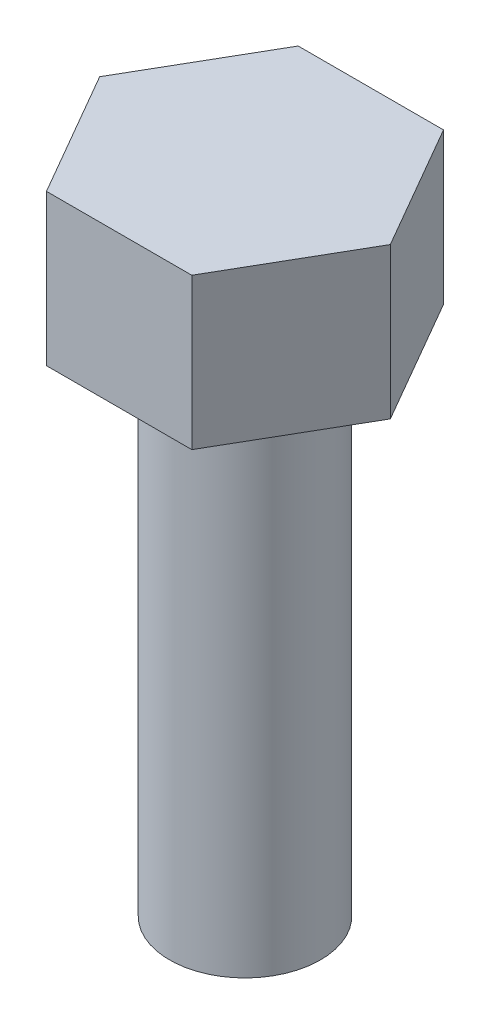
ISO-10303-21;
HEADER;
FILE_DESCRIPTION(('STEP AP214'),'2;1');
FILE_NAME('part.step','',(''),(''),'','','');
FILE_SCHEMA(('AUTOMOTIVE_DESIGN { 1 0 10303 214 1 1 1 1 }'));
ENDSEC;
DATA;
#1=APPLICATION_CONTEXT('core data for automotive mechanical design processes');
#2=APPLICATION_PROTOCOL_DEFINITION('international standard','automotive_design',2000,#1);
#3=PRODUCT_CONTEXT('',#1,'mechanical');
#4=PRODUCT('Part','Part','',(#3));
#5=PRODUCT_RELATED_PRODUCT_CATEGORY('part','',(#4));
#6=PRODUCT_DEFINITION_FORMATION('','',#4);
#7=PRODUCT_DEFINITION_CONTEXT('part definition',#1,'design');
#8=PRODUCT_DEFINITION('design','',#6,#7);
#9=PRODUCT_DEFINITION_SHAPE('','',#8);
#10=(LENGTH_UNIT() NAMED_UNIT(*) SI_UNIT(.MILLI.,.METRE.));
#11=(NAMED_UNIT(*) PLANE_ANGLE_UNIT() SI_UNIT($,.RADIAN.));
#12=(NAMED_UNIT(*) SI_UNIT($,.STERADIAN.) SOLID_ANGLE_UNIT());
#13=UNCERTAINTY_MEASURE_WITH_UNIT(LENGTH_MEASURE(1.E-05),#10,'distance_accuracy_value','');
#14=(GEOMETRIC_REPRESENTATION_CONTEXT(3) GLOBAL_UNCERTAINTY_ASSIGNED_CONTEXT((#13)) GLOBAL_UNIT_ASSIGNED_CONTEXT((#10,
#11,#12)) REPRESENTATION_CONTEXT('',''));
#15=CARTESIAN_POINT('',(0.,0.,0.));
#16=DIRECTION('',(0.,0.,1.));
#17=DIRECTION('',(1.,0.,0.));
#18=AXIS2_PLACEMENT_3D('',#15,#16,#17);
#19=CARTESIAN_POINT('',(1.44337567297406,3.,2.50000000000001));
#20=DIRECTION('',(-0.866025403784439,0.,-0.5));
#21=DIRECTION('',(-0.5,0.,0.866025403784439));
#22=AXIS2_PLACEMENT_3D('',#19,#20,#21);
#23=PLANE('',#22);
#24=DIRECTION('',(0.499999999999999,0.,-0.866025403784439));
#25=VECTOR('',#24,1.);
#26=CARTESIAN_POINT('',(1.44337567297406,0.,2.50000000000001));
#27=LINE('',#26,#25);
#28=CARTESIAN_POINT('',(1.44337567297406,0.,2.50000000000001));
#29=VERTEX_POINT('',#28);
#30=CARTESIAN_POINT('',(2.88675134594813,0.,0.));
#31=VERTEX_POINT('',#30);
#32=EDGE_CURVE('E124',#29,#31,#27,.T.);
#33=ORIENTED_EDGE('',*,*,#32,.T.);
#34=DIRECTION('',(0.,-1.,0.));
#35=VECTOR('',#34,1.);
#36=CARTESIAN_POINT('',(2.88675134594813,3.,0.));
#37=LINE('',#36,#35);
#38=CARTESIAN_POINT('',(2.88675134594813,3.,0.));
#39=VERTEX_POINT('',#38);
#40=EDGE_CURVE('E45',#39,#31,#37,.T.);
#41=ORIENTED_EDGE('',*,*,#40,.F.);
#42=DIRECTION('',(0.499999999999999,0.,-0.866025403784439));
#43=VECTOR('',#42,1.);
#44=CARTESIAN_POINT('',(1.44337567297406,3.,2.50000000000001));
#45=LINE('',#44,#43);
#46=CARTESIAN_POINT('',(1.44337567297406,3.,2.50000000000001));
#47=VERTEX_POINT('',#46);
#48=EDGE_CURVE('E138',#47,#39,#45,.T.);
#49=ORIENTED_EDGE('',*,*,#48,.F.);
#50=DIRECTION('',(0.,-1.,0.));
#51=VECTOR('',#50,1.);
#52=CARTESIAN_POINT('',(1.44337567297406,3.,2.50000000000001));
#53=LINE('',#52,#51);
#54=EDGE_CURVE('E123',#47,#29,#53,.T.);
#55=ORIENTED_EDGE('',*,*,#54,.T.);
#56=EDGE_LOOP('',(#33,#41,#49,#55));
#57=FACE_BOUND('',#56,.T.);
#58=ADVANCED_FACE('F39',(#57),#23,.F.);
#59=CARTESIAN_POINT('',(2.88675134594813,3.,0.));
#60=DIRECTION('',(-0.866025403784439,0.,0.5));
#61=DIRECTION('',(0.5,0.,0.866025403784439));
#62=AXIS2_PLACEMENT_3D('',#59,#60,#61);
#63=PLANE('',#62);
#64=DIRECTION('',(-0.5,0.,-0.866025403784438));
#65=VECTOR('',#64,1.);
#66=CARTESIAN_POINT('',(2.88675134594813,0.,0.));
#67=LINE('',#66,#65);
#68=CARTESIAN_POINT('',(1.44337567297406,0.,-2.50000000000001));
#69=VERTEX_POINT('',#68);
#70=EDGE_CURVE('E126',#31,#69,#67,.T.);
#71=ORIENTED_EDGE('',*,*,#70,.T.);
#72=DIRECTION('',(0.,-1.,0.));
#73=VECTOR('',#72,1.);
#74=CARTESIAN_POINT('',(1.44337567297406,3.,-2.50000000000001));
#75=LINE('',#74,#73);
#76=CARTESIAN_POINT('',(1.44337567297406,3.,-2.50000000000001));
#77=VERTEX_POINT('',#76);
#78=EDGE_CURVE('E137',#77,#69,#75,.T.);
#79=ORIENTED_EDGE('',*,*,#78,.F.);
#80=DIRECTION('',(-0.5,0.,-0.866025403784438));
#81=VECTOR('',#80,1.);
#82=CARTESIAN_POINT('',(2.88675134594813,3.,0.));
#83=LINE('',#82,#81);
#84=EDGE_CURVE('E94',#39,#77,#83,.T.);
#85=ORIENTED_EDGE('',*,*,#84,.F.);
#86=ORIENTED_EDGE('',*,*,#40,.T.);
#87=EDGE_LOOP('',(#71,#79,#85,#86));
#88=FACE_BOUND('',#87,.T.);
#89=ADVANCED_FACE('F145',(#88),#63,.F.);
#90=CARTESIAN_POINT('',(1.44337567297406,3.,-2.50000000000001));
#91=DIRECTION('',(0.,0.,1.));
#92=DIRECTION('',(1.,0.,0.));
#93=AXIS2_PLACEMENT_3D('',#90,#91,#92);
#94=PLANE('',#93);
#95=DIRECTION('',(-1.,0.,0.));
#96=VECTOR('',#95,1.);
#97=CARTESIAN_POINT('',(1.44337567297406,0.,-2.50000000000001));
#98=LINE('',#97,#96);
#99=CARTESIAN_POINT('',(-1.44337567297407,0.,-2.50000000000001));
#100=VERTEX_POINT('',#99);
#101=EDGE_CURVE('E131',#69,#100,#98,.T.);
#102=ORIENTED_EDGE('',*,*,#101,.T.);
#103=DIRECTION('',(0.,-1.,0.));
#104=VECTOR('',#103,1.);
#105=CARTESIAN_POINT('',(-1.44337567297407,3.,-2.50000000000001));
#106=LINE('',#105,#104);
#107=CARTESIAN_POINT('',(-1.44337567297407,3.,-2.50000000000001));
#108=VERTEX_POINT('',#107);
#109=EDGE_CURVE('E116',#108,#100,#106,.T.);
#110=ORIENTED_EDGE('',*,*,#109,.F.);
#111=DIRECTION('',(-1.,0.,0.));
#112=VECTOR('',#111,1.);
#113=CARTESIAN_POINT('',(1.44337567297406,3.,-2.50000000000001));
#114=LINE('',#113,#112);
#115=EDGE_CURVE('E110',#77,#108,#114,.T.);
#116=ORIENTED_EDGE('',*,*,#115,.F.);
#117=ORIENTED_EDGE('',*,*,#78,.T.);
#118=EDGE_LOOP('',(#102,#110,#116,#117));
#119=FACE_BOUND('',#118,.T.);
#120=ADVANCED_FACE('F147',(#119),#94,.F.);
#121=CARTESIAN_POINT('',(-1.44337567297407,3.,-2.50000000000001));
#122=DIRECTION('',(0.866025403784439,0.,0.5));
#123=DIRECTION('',(0.5,0.,-0.866025403784439));
#124=AXIS2_PLACEMENT_3D('',#121,#122,#123);
#125=PLANE('',#124);
#126=DIRECTION('',(-0.5,0.,0.866025403784439));
#127=VECTOR('',#126,1.);
#128=CARTESIAN_POINT('',(-1.44337567297407,0.,-2.50000000000001));
#129=LINE('',#128,#127);
#130=CARTESIAN_POINT('',(-2.88675134594813,0.,0.));
#131=VERTEX_POINT('',#130);
#132=EDGE_CURVE('E113',#100,#131,#129,.T.);
#133=ORIENTED_EDGE('',*,*,#132,.T.);
#134=DIRECTION('',(0.,-1.,0.));
#135=VECTOR('',#134,1.);
#136=CARTESIAN_POINT('',(-2.88675134594813,3.,0.));
#137=LINE('',#136,#135);
#138=CARTESIAN_POINT('',(-2.88675134594813,3.,0.));
#139=VERTEX_POINT('',#138);
#140=EDGE_CURVE('E115',#139,#131,#137,.T.);
#141=ORIENTED_EDGE('',*,*,#140,.F.);
#142=DIRECTION('',(-0.5,0.,0.866025403784439));
#143=VECTOR('',#142,1.);
#144=CARTESIAN_POINT('',(-1.44337567297407,3.,-2.50000000000001));
#145=LINE('',#144,#143);
#146=EDGE_CURVE('E101',#108,#139,#145,.T.);
#147=ORIENTED_EDGE('',*,*,#146,.F.);
#148=ORIENTED_EDGE('',*,*,#109,.T.);
#149=EDGE_LOOP('',(#133,#141,#147,#148));
#150=FACE_BOUND('',#149,.T.);
#151=ADVANCED_FACE('F114',(#150),#125,.F.);
#152=CARTESIAN_POINT('',(-2.88675134594813,3.,0.));
#153=DIRECTION('',(0.866025403784439,0.,-0.5));
#154=DIRECTION('',(-0.5,0.,-0.866025403784439));
#155=AXIS2_PLACEMENT_3D('',#152,#153,#154);
#156=PLANE('',#155);
#157=DIRECTION('',(0.5,0.,0.866025403784439));
#158=VECTOR('',#157,1.);
#159=CARTESIAN_POINT('',(-2.88675134594813,0.,0.));
#160=LINE('',#159,#158);
#161=CARTESIAN_POINT('',(-1.44337567297407,0.,2.5));
#162=VERTEX_POINT('',#161);
#163=EDGE_CURVE('E78',#131,#162,#160,.T.);
#164=ORIENTED_EDGE('',*,*,#163,.T.);
#165=DIRECTION('',(0.,-1.,0.));
#166=VECTOR('',#165,1.);
#167=CARTESIAN_POINT('',(-1.44337567297407,3.,2.5));
#168=LINE('',#167,#166);
#169=CARTESIAN_POINT('',(-1.44337567297407,3.,2.5));
#170=VERTEX_POINT('',#169);
#171=EDGE_CURVE('E117',#170,#162,#168,.T.);
#172=ORIENTED_EDGE('',*,*,#171,.F.);
#173=DIRECTION('',(0.5,0.,0.866025403784439));
#174=VECTOR('',#173,1.);
#175=CARTESIAN_POINT('',(-2.88675134594813,3.,0.));
#176=LINE('',#175,#174);
#177=EDGE_CURVE('E104',#139,#170,#176,.T.);
#178=ORIENTED_EDGE('',*,*,#177,.F.);
#179=ORIENTED_EDGE('',*,*,#140,.T.);
#180=EDGE_LOOP('',(#164,#172,#178,#179));
#181=FACE_BOUND('',#180,.T.);
#182=ADVANCED_FACE('F118',(#181),#156,.F.);
#183=CARTESIAN_POINT('',(-1.44337567297407,3.,2.5));
#184=DIRECTION('',(0.,0.,-1.));
#185=DIRECTION('',(-1.,0.,0.));
#186=AXIS2_PLACEMENT_3D('',#183,#184,#185);
#187=PLANE('',#186);
#188=DIRECTION('',(1.,0.,0.));
#189=VECTOR('',#188,1.);
#190=CARTESIAN_POINT('',(-1.44337567297407,0.,2.5));
#191=LINE('',#190,#189);
#192=EDGE_CURVE('E84',#162,#29,#191,.T.);
#193=ORIENTED_EDGE('',*,*,#192,.T.);
#194=ORIENTED_EDGE('',*,*,#54,.F.);
#195=DIRECTION('',(1.,0.,0.));
#196=VECTOR('',#195,1.);
#197=CARTESIAN_POINT('',(-1.44337567297407,3.,2.5));
#198=LINE('',#197,#196);
#199=EDGE_CURVE('E57',#170,#47,#198,.T.);
#200=ORIENTED_EDGE('',*,*,#199,.F.);
#201=ORIENTED_EDGE('',*,*,#171,.T.);
#202=EDGE_LOOP('',(#193,#194,#200,#201));
#203=FACE_BOUND('',#202,.T.);
#204=ADVANCED_FACE('F168',(#203),#187,.F.);
#205=CARTESIAN_POINT('',(0.,3.,0.));
#206=DIRECTION('',(0.,1.,0.));
#207=DIRECTION('',(0.,0.,1.));
#208=AXIS2_PLACEMENT_3D('',#205,#206,#207);
#209=PLANE('',#208);
#210=ORIENTED_EDGE('',*,*,#48,.T.);
#211=ORIENTED_EDGE('',*,*,#84,.T.);
#212=ORIENTED_EDGE('',*,*,#115,.T.);
#213=ORIENTED_EDGE('',*,*,#146,.T.);
#214=ORIENTED_EDGE('',*,*,#177,.T.);
#215=ORIENTED_EDGE('',*,*,#199,.T.);
#216=EDGE_LOOP('',(#210,#211,#212,#213,#214,#215));
#217=FACE_BOUND('',#216,.T.);
#218=ADVANCED_FACE('F103',(#217),#209,.T.);
#219=CARTESIAN_POINT('',(0.,0.,0.));
#220=DIRECTION('',(0.,1.,0.));
#221=DIRECTION('',(0.,0.,1.));
#222=AXIS2_PLACEMENT_3D('',#219,#220,#221);
#223=PLANE('',#222);
#224=CARTESIAN_POINT('',(0.,0.,0.));
#225=DIRECTION('',(0.,-1.,0.));
#226=DIRECTION('',(0.,0.,-1.));
#227=AXIS2_PLACEMENT_3D('',#224,#225,#226);
#228=CIRCLE('',#227,1.5);
#229=CARTESIAN_POINT('',(0.,0.,-1.5));
#230=VERTEX_POINT('',#229);
#231=EDGE_CURVE('E11',#230,#230,#228,.T.);
#232=ORIENTED_EDGE('',*,*,#231,.F.);
#233=EDGE_LOOP('',(#232));
#234=FACE_BOUND('',#233,.T.);
#235=ORIENTED_EDGE('',*,*,#32,.F.);
#236=ORIENTED_EDGE('',*,*,#192,.F.);
#237=ORIENTED_EDGE('',*,*,#163,.F.);
#238=ORIENTED_EDGE('',*,*,#132,.F.);
#239=ORIENTED_EDGE('',*,*,#101,.F.);
#240=ORIENTED_EDGE('',*,*,#70,.F.);
#241=EDGE_LOOP('',(#235,#236,#237,#238,#239,#240));
#242=FACE_BOUND('',#241,.T.);
#243=ADVANCED_FACE('F149',(#234,#242),#223,.F.);
#244=CARTESIAN_POINT('',(0.,-10.,0.));
#245=DIRECTION('',(0.,1.,0.));
#246=DIRECTION('',(0.,0.,1.));
#247=AXIS2_PLACEMENT_3D('',#244,#245,#246);
#248=CYLINDRICAL_SURFACE('',#247,1.5);
#249=CARTESIAN_POINT('',(0.,-10.,0.));
#250=DIRECTION('',(0.,-1.,0.));
#251=DIRECTION('',(0.,0.,-1.));
#252=AXIS2_PLACEMENT_3D('',#249,#250,#251);
#253=CIRCLE('',#252,1.5);
#254=CARTESIAN_POINT('',(0.,-10.,-1.5));
#255=VERTEX_POINT('',#254);
#256=EDGE_CURVE('E129',#255,#255,#253,.T.);
#257=ORIENTED_EDGE('',*,*,#256,.F.);
#258=EDGE_LOOP('',(#257));
#259=FACE_BOUND('',#258,.T.);
#260=ORIENTED_EDGE('',*,*,#231,.T.);
#261=EDGE_LOOP('',(#260));
#262=FACE_BOUND('',#261,.T.);
#263=ADVANCED_FACE('F157',(#259,#262),#248,.T.);
#264=CARTESIAN_POINT('',(0.,-10.,0.));
#265=DIRECTION('',(0.,-1.,0.));
#266=DIRECTION('',(0.,0.,-1.));
#267=AXIS2_PLACEMENT_3D('',#264,#265,#266);
#268=PLANE('',#267);
#269=ORIENTED_EDGE('',*,*,#256,.T.);
#270=EDGE_LOOP('',(#269));
#271=FACE_BOUND('',#270,.T.);
#272=ADVANCED_FACE('F160',(#271),#268,.T.);
#273=CLOSED_SHELL('',(#58,#89,#120,#151,#182,#204,#218,#243,#263,#272));
#274=MANIFOLD_SOLID_BREP('B2',#273);
#275=ADVANCED_BREP_SHAPE_REPRESENTATION('',(#18,#274),#14);
#276=SHAPE_DEFINITION_REPRESENTATION(#9,#275);
ENDSEC;
END-ISO-10303-21;
